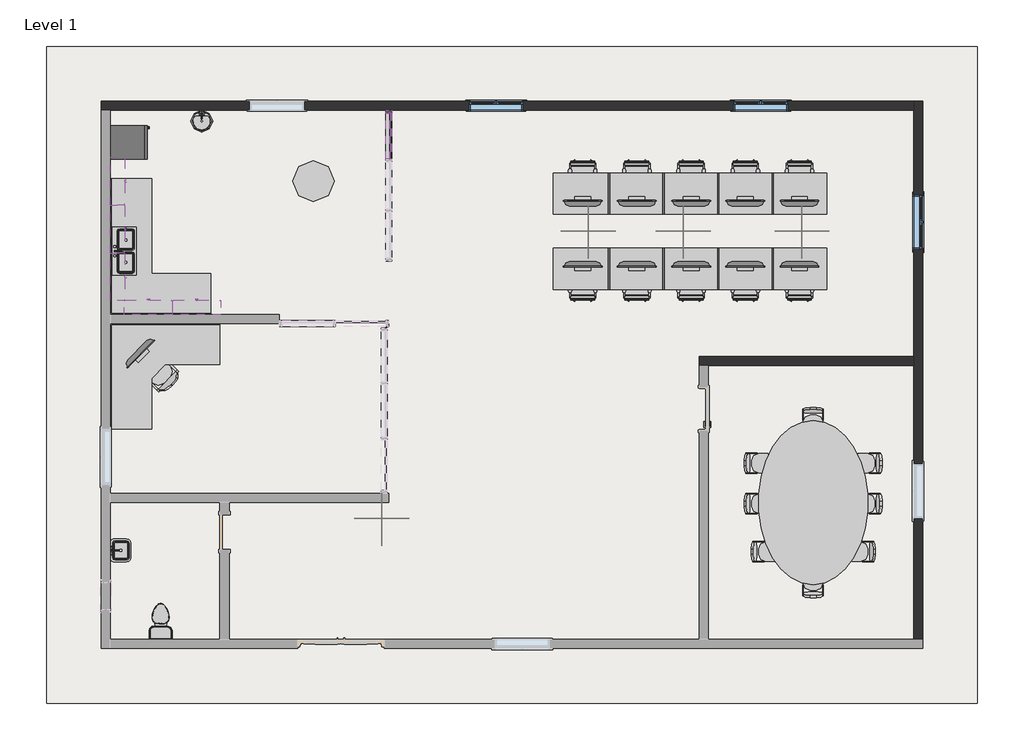
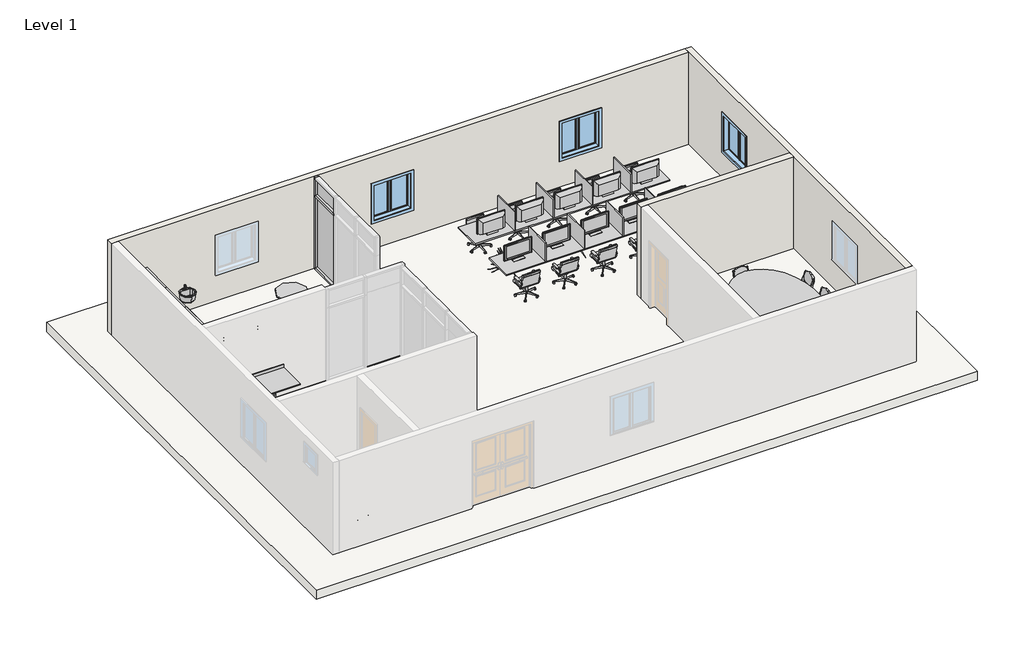
# One storey, part 2 of 2: 43 furniture elements, 10 plates, 4 flow terminals, 4 geographic elements, 4 members, 3 walls, 3 windows, 1 proxy, 1 slab.
"""IFC4 building model written with IfcOpenShell, lengths in millimetres."""

from ifc_helpers import new_model, si_unit, frame, origin, place, context, project, spatial, polyline, outline, extrude, faceted_brep, transform, mapped, element, save
from components import proxy_a13a33b2, flow_terminal_a53be723, flow_terminal_d49f872f, flow_terminal_62a433f7, toilet_domestic_3d_toilet_domestic_3d_f7549cf7, toilet_domestic_3d_toilet_domestic_3d_183bbd19, furniture_2d7fc6e7, chair_executive_chair_executive_8d69e98c, chair_task_arms_chair_task_arms_fa5a08ef, furniture_cfc005fb, furniture_c973ddc6, furniture_51338070, furniture_3d1d9cbc, furniture_2ec127df, furniture_56245f3a, furniture_905aceb5, furniture_1a6705e8, furniture_7e2871f8, rpc_plant_tropical_agave_1_5_74a88192, member_47bfaf8a, member_ee409385, member_a1c24a98, member_38455fd9, system_panel_glazed_82e05715, system_panel_glazed_958d1135, system_panel_glazed_6663e6a9, window_0862ab64

model = new_model("IFC4")

# Units and contexts
model_context = context("Model", 3, world=origin())
ifc_project = project(units=[si_unit("LENGTHUNIT", "METRE", prefix="MILLI")], contexts=[model_context])

# Site, building, storey
site = spatial("IfcSite", under=ifc_project)
building = spatial("IfcBuilding", under=site)
storey = spatial("IfcBuildingStorey", under=building, Name="Level 1", Elevation=0.0)

# Proxy
placement = place(None, origin())
proxy_shape = proxy_a13a33b2(model_context)
element("IfcBuildingElementProxy", 1, Name="Refrigerator : 30\" x 32\" RH", ObjectType="Refrigerator : 30\" x 32\" RH", at=placement, inside=storey, context=model_context, shape_type="MappedRepresentation", body=[
    mapped(proxy_shape, transform((-15846.011402, 5252.7824508, 0.0), x_axis=(0.0, 1.0000000000000002, 0.0), y_axis=(-1.0000000000000002, 0.0, 0.0), z_axis=(0.0, 0.0, 1.0))),
])

# Flow terminals
flow_terminal_shape = flow_terminal_a53be723(model_context)
element("IfcFlowTerminal", 2, ObjectType="Sink Kitchen-Double : 42\" x 21\"", at=placement, inside=storey, context=model_context, shape_type="MappedRepresentation", body=[
    mapped(flow_terminal_shape, transform((-15937.3285008, 2818.9421817, 0.0), x_axis=(0.0, 1.0000000000000002, 0.0), y_axis=(-1.0000000000000002, 0.0, 0.0), z_axis=(0.0, 0.0, 1.0))),
])
flow_terminal_2_shape = flow_terminal_d49f872f(model_context)
element("IfcFlowTerminal", 3, ObjectType="Sink Vanity-Round : 19\" x 19\"", at=placement, inside=storey, context=model_context, shape_type="MappedRepresentation", body=[
    mapped(flow_terminal_2_shape, transform((-14309.1256425, 5647.2327419, 0.0), x_axis=(1.0, 0.0, 0.0), y_axis=(0.0, 1.0, 0.0), z_axis=(0.0, 0.0, 1.0))),
])
flow_terminal_3_shape = flow_terminal_62a433f7(model_context)
element("IfcFlowTerminal", 4, ObjectType="Sink Vanity-Square : 20\" x 18\"", at=placement, inside=storey, context=model_context, shape_type="MappedRepresentation", body=[
    mapped(flow_terminal_3_shape, transform((-16064.3285008, -3848.5578183, 0.0), x_axis=(0.0, 1.0000000000000002, 0.0), y_axis=(-1.0000000000000002, 0.0, 0.0), z_axis=(0.0, 0.0, 1.0))),
])
toilet_domestic_3d_toilet_domestic_3d_shape = toilet_domestic_3d_toilet_domestic_3d_f7549cf7(model_context)
toilet_domestic_3d_toilet_domestic_3d_2_shape = toilet_domestic_3d_toilet_domestic_3d_183bbd19(model_context)
element("IfcFlowTerminal", 5, ObjectType="Toilet-Domestic-3D : Toilet-Domestic-3D", at=placement, inside=storey, context=model_context, shape_type="MappedRepresentation", body=[
    mapped(toilet_domestic_3d_toilet_domestic_3d_shape, transform((-15126.873902, -5319.3725504, 0.0), x_axis=(-1.0000000000000004, 0.0, 0.0), y_axis=(0.0, -1.0000000000000004, 0.0), z_axis=(0.0, 0.0, 1.0))),
    mapped(toilet_domestic_3d_toilet_domestic_3d_2_shape, transform((-15126.873902, -5319.3725504, 0.0), x_axis=(-1.0000000000000004, 0.0, 0.0), y_axis=(0.0, -1.0000000000000004, 0.0), z_axis=(0.0, 0.0, 1.0))),
])

# Furniture
furniture_shape = furniture_2d7fc6e7(model_context)
element("IfcFurniture", 6, ObjectType="48\"", at=placement, inside=storey, context=model_context, shape_type="MappedRepresentation", body=[
    mapped(furniture_shape, transform((-14655.028942, 1424.9314222, 0.0), x_axis=(-1.0000000000000004, 0.0, 0.0), y_axis=(0.0, -1.0000000000000004, 0.0), z_axis=(0.0, 0.0, 1.0))),
])
element("IfcFurniture", 7, ObjectType="48\"", at=placement, inside=storey, context=model_context, shape_type="MappedRepresentation", body=[
    mapped(furniture_shape, transform((-16193.673902, 3772.4864623, 0.0), x_axis=(0.0, 1.0000000000000002, 0.0), y_axis=(-1.0000000000000002, 0.0, 0.0), z_axis=(0.0, 0.0, 1.0))),
])
chair_executive_chair_executive_shape = chair_executive_chair_executive_8d69e98c(model_context)
element("IfcFurniture", 8, ObjectType="Chair-Executive : Chair-Executive", at=placement, inside=storey, context=model_context, shape_type="MappedRepresentation", body=[
    mapped(chair_executive_chair_executive_shape, transform((-15213.1726911, -8.960918, 0.0), x_axis=(0.7071067811865517, 0.707106781186545, 0.0), y_axis=(-0.707106781186545, 0.7071067811865517, 0.0), z_axis=(0.0, 0.0, 1.0))),
])
chair_task_arms_chair_task_arms_shape = chair_task_arms_chair_task_arms_fa5a08ef(model_context)
element("IfcFurniture", 9, ObjectType="Chair-Task Arms : Chair-Task Arms", at=placement, inside=storey, context=model_context, shape_type="MappedRepresentation", body=[
    mapped(chair_task_arms_chair_task_arms_shape, transform((-5587.8830823, 4593.4773239, 0.0), x_axis=(-1.0000000000000004, 0.0, 0.0), y_axis=(0.0, -1.0000000000000004, 0.0), z_axis=(0.0, 0.0, 1.0))),
])
element("IfcFurniture", 10, ObjectType="Chair-Task Arms : Chair-Task Arms", at=placement, inside=storey, context=model_context, shape_type="MappedRepresentation", body=[
    mapped(chair_task_arms_chair_task_arms_shape, transform((-5869.8647216, 1990.1855206, 0.0), x_axis=(1.0000000000000002, 0.0, 0.0), y_axis=(0.0, 1.0000000000000002, 0.0), z_axis=(0.0, 0.0, 1.0))),
])
element("IfcFurniture", 11, ObjectType="Chair-Task Arms : Chair-Task Arms", at=placement, inside=storey, context=model_context, shape_type="MappedRepresentation", body=[
    mapped(chair_task_arms_chair_task_arms_shape, transform((-761.8830823, 4593.4773239, 0.0), x_axis=(-1.0, 0.0, 0.0), y_axis=(0.0, -1.0, 0.0), z_axis=(0.0, 0.0, 1.0))),
])
element("IfcFurniture", 12, ObjectType="Chair-Task Arms : Chair-Task Arms", at=placement, inside=storey, context=model_context, shape_type="MappedRepresentation", body=[
    mapped(chair_task_arms_chair_task_arms_shape, transform((-1043.8647216, 1990.1855206, 0.0), x_axis=(1.0, 0.0, 0.0), y_axis=(0.0, 1.0, 0.0), z_axis=(0.0, 0.0, 1.0))),
])
element("IfcFurniture", 13, ObjectType="Chair-Task Arms : Chair-Task Arms", at=placement, inside=storey, context=model_context, shape_type="MappedRepresentation", body=[
    mapped(chair_task_arms_chair_task_arms_shape, transform((-4381.3830823, 4593.4773239, 0.0), x_axis=(-1.0, 0.0, 0.0), y_axis=(0.0, -1.0, 0.0), z_axis=(0.0, 0.0, 1.0))),
])
element("IfcFurniture", 14, ObjectType="Chair-Task Arms : Chair-Task Arms", at=placement, inside=storey, context=model_context, shape_type="MappedRepresentation", body=[
    mapped(chair_task_arms_chair_task_arms_shape, transform((-4663.3647216, 1990.1855206, 0.0), x_axis=(1.0, 0.0, 0.0), y_axis=(0.0, 1.0, 0.0), z_axis=(0.0, 0.0, 1.0))),
])
element("IfcFurniture", 15, ObjectType="Chair-Task Arms : Chair-Task Arms", at=placement, inside=storey, context=model_context, shape_type="MappedRepresentation", body=[
    mapped(chair_task_arms_chair_task_arms_shape, transform((-3174.8830823, 4593.4773239, 0.0), x_axis=(-1.0, 0.0, 0.0), y_axis=(0.0, -1.0, 0.0), z_axis=(0.0, 0.0, 1.0))),
])
element("IfcFurniture", 16, ObjectType="Chair-Task Arms : Chair-Task Arms", at=placement, inside=storey, context=model_context, shape_type="MappedRepresentation", body=[
    mapped(chair_task_arms_chair_task_arms_shape, transform((-3456.8647216, 1990.1855206, 0.0), x_axis=(1.0, 0.0, 0.0), y_axis=(0.0, 1.0, 0.0), z_axis=(0.0, 0.0, 1.0))),
])
element("IfcFurniture", 17, ObjectType="Chair-Task Arms : Chair-Task Arms", at=placement, inside=storey, context=model_context, shape_type="MappedRepresentation", body=[
    mapped(chair_task_arms_chair_task_arms_shape, transform((-1968.3830823, 4593.4773239, 0.0), x_axis=(-1.0, 0.0, 0.0), y_axis=(0.0, -1.0, 0.0), z_axis=(0.0, 0.0, 1.0))),
])
element("IfcFurniture", 18, ObjectType="Chair-Task Arms : Chair-Task Arms", at=placement, inside=storey, context=model_context, shape_type="MappedRepresentation", body=[
    mapped(chair_task_arms_chair_task_arms_shape, transform((-2250.3647216, 1990.1855206, 0.0), x_axis=(1.0, 0.0, 0.0), y_axis=(0.0, 1.0, 0.0), z_axis=(0.0, 0.0, 1.0))),
])
furniture_2_shape = furniture_cfc005fb(model_context)
element("IfcFurniture", 19, ObjectType="Counter Top-Island : 48\" Depth", at=placement, inside=storey, context=model_context, shape_type="MappedRepresentation", body=[
    mapped(furniture_2_shape, transform((-5188.8116069, 4549.1314222, 914.4), x_axis=(1.0, 0.0, 0.0), y_axis=(0.0, 1.0, 0.0), z_axis=(0.0, 0.0, 1.0))),
])
element("IfcFurniture", 20, ObjectType="Counter Top-Island : 48\" Depth", at=placement, inside=storey, context=model_context, shape_type="MappedRepresentation", body=[
    mapped(furniture_2_shape, transform((-5188.8116069, 2872.7314222, 914.4), x_axis=(1.0, 0.0, 0.0), y_axis=(0.0, 1.0, 0.0), z_axis=(0.0, 0.0, 1.0))),
])
furniture_3_shape = furniture_c973ddc6(model_context)
element("IfcFurniture", 21, ObjectType="Counter Top-L Shaped 2 : 24\" Depth", at=placement, inside=storey, context=model_context, shape_type="MappedRepresentation", body=[
    mapped(furniture_3_shape, transform((-15044.0116069, 1221.7314222, 0.0), x_axis=(1.0, 0.0, 0.0), y_axis=(0.0, 1.0, 0.0), z_axis=(0.0, 0.0, 1.0))),
])
furniture_4_shape = furniture_51338070(model_context)
element("IfcFurniture", 22, ObjectType="Counter Top-L Shaped w Sink : 24\" Depth", at=placement, inside=storey, context=model_context, shape_type="MappedRepresentation", body=[
    mapped(furniture_4_shape, transform((-16244.473902, 2625.3937173, 0.0), x_axis=(0.0, 1.0000000000000002, 0.0), y_axis=(-1.0000000000000002, 0.0, 0.0), z_axis=(0.0, 0.0, 1.0))),
])
furniture_5_shape = furniture_3d1d9cbc(model_context)
element("IfcFurniture", 23, ObjectType="Seating-Auditorium : 18\" x 24\" x 30\"", at=placement, inside=storey, context=model_context, shape_type="MappedRepresentation", body=[
    mapped(furniture_5_shape, transform((-1880.1493118, -3697.5407089, 0.0), x_axis=(0.0, -1.0000000000000004, 0.0), y_axis=(1.0000000000000004, 0.0, 0.0), z_axis=(0.0, 0.0, 1.0))),
])
element("IfcFurniture", 24, ObjectType="Seating-Auditorium : 18\" x 24\" x 30\"", at=placement, inside=storey, context=model_context, shape_type="MappedRepresentation", body=[
    mapped(furniture_5_shape, transform((-2032.5493118, -2630.7407089, 0.0), x_axis=(0.0, -1.0, 0.0), y_axis=(1.0, 0.0, 0.0), z_axis=(0.0, 0.0, 1.0))),
])
element("IfcFurniture", 25, ObjectType="Seating-Auditorium : 18\" x 24\" x 30\"", at=placement, inside=storey, context=model_context, shape_type="MappedRepresentation", body=[
    mapped(furniture_5_shape, transform((-2032.5493118, -1729.0407089, 0.0), x_axis=(0.0, -1.0, 0.0), y_axis=(1.0, 0.0, 0.0), z_axis=(0.0, 0.0, 1.0))),
])
element("IfcFurniture", 26, ObjectType="Seating-Auditorium : 18\" x 24\" x 30\"", at=placement, inside=storey, context=model_context, shape_type="MappedRepresentation", body=[
    mapped(furniture_5_shape, transform((-437.3460331, -747.3931679, 0.0), x_axis=(-1.0000000000000002, 0.0, 0.0), y_axis=(0.0, -1.0000000000000002, 0.0), z_axis=(0.0, 0.0, 1.0))),
])
element("IfcFurniture", 27, ObjectType="Seating-Auditorium : 18\" x 24\" x 30\"", at=placement, inside=storey, context=model_context, shape_type="MappedRepresentation", body=[
    mapped(furniture_5_shape, transform((-758.8017708, -4784.7439876, 0.0), x_axis=(1.0000000000000002, 0.0, 0.0), y_axis=(0.0, 1.0000000000000002, 0.0), z_axis=(0.0, 0.0, 1.0))),
])
furniture_6_shape = furniture_2ec127df(model_context)
element("IfcFurniture", 28, ObjectType="Seating-Auditorium : 18\" x 24\" x 30\"", at=placement, inside=storey, context=model_context, shape_type="MappedRepresentation", body=[
    mapped(furniture_6_shape, transform((684.0015079, -3697.5407089, 0.0), x_axis=(0.0, -1.0000000000000004, 0.0), y_axis=(1.0000000000000004, 0.0, 0.0), z_axis=(0.0, 0.0, 1.0))),
])
element("IfcFurniture", 29, ObjectType="Seating-Auditorium : 18\" x 24\" x 30\"", at=placement, inside=storey, context=model_context, shape_type="MappedRepresentation", body=[
    mapped(furniture_6_shape, transform((836.4015079, -2630.7407089, 0.0), x_axis=(0.0, -1.0, 0.0), y_axis=(1.0, 0.0, 0.0), z_axis=(0.0, 0.0, 1.0))),
])
element("IfcFurniture", 30, ObjectType="Seating-Auditorium : 18\" x 24\" x 30\"", at=placement, inside=storey, context=model_context, shape_type="MappedRepresentation", body=[
    mapped(furniture_6_shape, transform((836.4015079, -1729.0407089, 0.0), x_axis=(0.0, -1.0, 0.0), y_axis=(1.0, 0.0, 0.0), z_axis=(0.0, 0.0, 1.0))),
])
furniture_7_shape = furniture_56245f3a(model_context)
element("IfcFurniture", 31, ObjectType="TV - Flat Screen : 32\"", at=placement, inside=storey, context=model_context, shape_type="MappedRepresentation", body=[
    mapped(furniture_7_shape, transform((-15605.6880737, 588.5239794, 914.4), x_axis=(0.7071067811865503, 0.7071067811865462, 0.0), y_axis=(-0.7071067811865462, 0.7071067811865503, 0.0), z_axis=(0.0, 0.0, 1.0))),
])
element("IfcFurniture", 32, ObjectType="TV - Flat Screen : 32\"", at=placement, inside=storey, context=model_context, shape_type="MappedRepresentation", body=[
    mapped(furniture_7_shape, transform((-5732.8184161, 3898.7406257, 914.4), x_axis=(-1.0000000000000004, 0.0, 0.0), y_axis=(0.0, -1.0000000000000004, 0.0), z_axis=(0.0, 0.0, 1.0))),
])
element("IfcFurniture", 33, ObjectType="TV - Flat Screen : 32\"", at=placement, inside=storey, context=model_context, shape_type="MappedRepresentation", body=[
    mapped(furniture_7_shape, transform((-5724.9293878, 2548.0551491, 914.4), x_axis=(1.0000000000000002, 0.0, 0.0), y_axis=(0.0, 1.0000000000000002, 0.0), z_axis=(0.0, 0.0, 1.0))),
])
element("IfcFurniture", 34, ObjectType="TV - Flat Screen : 32\"", at=placement, inside=storey, context=model_context, shape_type="MappedRepresentation", body=[
    mapped(furniture_7_shape, transform((-906.8184161, 3898.7406257, 914.4), x_axis=(-1.0, 0.0, 0.0), y_axis=(0.0, -1.0, 0.0), z_axis=(0.0, 0.0, 1.0))),
])
element("IfcFurniture", 35, ObjectType="TV - Flat Screen : 32\"", at=placement, inside=storey, context=model_context, shape_type="MappedRepresentation", body=[
    mapped(furniture_7_shape, transform((-898.9293878, 2548.0551491, 914.4), x_axis=(1.0, 0.0, 0.0), y_axis=(0.0, 1.0, 0.0), z_axis=(0.0, 0.0, 1.0))),
])
element("IfcFurniture", 36, ObjectType="TV - Flat Screen : 32\"", at=placement, inside=storey, context=model_context, shape_type="MappedRepresentation", body=[
    mapped(furniture_7_shape, transform((-4526.3184161, 3898.7406257, 914.4), x_axis=(-1.0, 0.0, 0.0), y_axis=(0.0, -1.0, 0.0), z_axis=(0.0, 0.0, 1.0))),
])
element("IfcFurniture", 37, ObjectType="TV - Flat Screen : 32\"", at=placement, inside=storey, context=model_context, shape_type="MappedRepresentation", body=[
    mapped(furniture_7_shape, transform((-4518.4293878, 2548.0551491, 914.4), x_axis=(1.0, 0.0, 0.0), y_axis=(0.0, 1.0, 0.0), z_axis=(0.0, 0.0, 1.0))),
])
element("IfcFurniture", 38, ObjectType="TV - Flat Screen : 32\"", at=placement, inside=storey, context=model_context, shape_type="MappedRepresentation", body=[
    mapped(furniture_7_shape, transform((-3319.8184161, 3898.7406257, 914.4), x_axis=(-1.0, 0.0, 0.0), y_axis=(0.0, -1.0, 0.0), z_axis=(0.0, 0.0, 1.0))),
])
element("IfcFurniture", 39, ObjectType="TV - Flat Screen : 32\"", at=placement, inside=storey, context=model_context, shape_type="MappedRepresentation", body=[
    mapped(furniture_7_shape, transform((-3311.9293878, 2548.0551491, 914.4), x_axis=(1.0, 0.0, 0.0), y_axis=(0.0, 1.0, 0.0), z_axis=(0.0, 0.0, 1.0))),
])
element("IfcFurniture", 40, ObjectType="TV - Flat Screen : 32\"", at=placement, inside=storey, context=model_context, shape_type="MappedRepresentation", body=[
    mapped(furniture_7_shape, transform((-2113.3184161, 3898.7406257, 914.4), x_axis=(-1.0, 0.0, 0.0), y_axis=(0.0, -1.0, 0.0), z_axis=(0.0, 0.0, 1.0))),
])
element("IfcFurniture", 41, ObjectType="TV - Flat Screen : 32\"", at=placement, inside=storey, context=model_context, shape_type="MappedRepresentation", body=[
    mapped(furniture_7_shape, transform((-2105.4293878, 2548.0551491, 914.4), x_axis=(1.0, 0.0, 0.0), y_axis=(0.0, 1.0, 0.0), z_axis=(0.0, 0.0, 1.0))),
])
furniture_8_shape = furniture_905aceb5(model_context)
element("IfcFurniture", 42, ObjectType="Table-Dining Round w Chairs : 36\" Diameter", at=placement, inside=storey, context=model_context, shape_type="MappedRepresentation", body=[
    mapped(furniture_8_shape, transform((-11826.9558692, 4581.6101108, 0.0), x_axis=(1.0, 0.0, 0.0), y_axis=(0.0, 1.0, 0.0), z_axis=(0.0, 0.0, 1.0))),
])
furniture_9_shape = furniture_1a6705e8(model_context)
element("IfcFurniture", 43, ObjectType="Table-Ellipse : 72\" x 36\"", at=placement, inside=storey, context=model_context, shape_type="MappedRepresentation", body=[
    mapped(furniture_9_shape, transform((-598.073902, -2766.0685778, 0.0), x_axis=(0.0, 1.0, 0.0), y_axis=(-1.0, 0.0, 0.0), z_axis=(0.0, 0.0, 1.0))),
])
furniture_10_shape = furniture_7e2871f8(model_context)
element("IfcFurniture", 44, ObjectType="Upper Cabinet-Double Door-Wall : 42\"", at=placement, inside=storey, context=model_context, shape_type="MappedRepresentation", body=[
    mapped(furniture_10_shape, transform((-16346.073902, 2292.902585, 573.9321915), x_axis=(0.0, -1.0, 0.0), y_axis=(1.0, 0.0, 0.0), z_axis=(0.0, 0.0, 1.0))),
])
element("IfcFurniture", 45, ObjectType="Upper Cabinet-Double Door-Wall : 42\"", at=placement, inside=storey, context=model_context, shape_type="MappedRepresentation", body=[
    mapped(furniture_10_shape, transform((-16346.073902, 4426.502585, 573.9321915), x_axis=(0.0, -1.0, 0.0), y_axis=(1.0, 0.0, 0.0), z_axis=(0.0, 0.0, 1.0))),
])
element("IfcFurniture", 46, ObjectType="Upper Cabinet-Double Door-Wall : 42\"", at=placement, inside=storey, context=model_context, shape_type="MappedRepresentation", body=[
    mapped(furniture_10_shape, transform((-16346.073902, 3359.702585, 573.9321915), x_axis=(0.0, -1.0, 0.0), y_axis=(1.0, 0.0, 0.0), z_axis=(0.0, 0.0, 1.0))),
])
element("IfcFurniture", 47, ObjectType="Upper Cabinet-Double Door-Wall : 42\"", at=placement, inside=storey, context=model_context, shape_type="MappedRepresentation", body=[
    mapped(furniture_10_shape, transform((-15429.6950647, 1323.3314222, 588.7403508), x_axis=(1.0, 0.0, 0.0), y_axis=(0.0, 1.0, 0.0), z_axis=(0.0, 0.0, 1.0))),
])
element("IfcFurniture", 48, ObjectType="Upper Cabinet-Double Door-Wall : 42\"", at=placement, inside=storey, context=model_context, shape_type="MappedRepresentation", body=[
    mapped(furniture_10_shape, transform((-14356.5450647, 1323.3314222, 588.7403508), x_axis=(1.0, 0.0, 0.0), y_axis=(0.0, 1.0, 0.0), z_axis=(0.0, 0.0, 1.0))),
])

# Geographic elements
rpc_plant_tropical_agave_1_5_shape = rpc_plant_tropical_agave_1_5_74a88192(model_context)
element("IfcGeographicElement", 49, ObjectType="RPC Plant - Tropical : Agave - 1.5'", at=placement, inside=storey, context=model_context, shape_type="MappedRepresentation", body=[
    mapped(rpc_plant_tropical_agave_1_5_shape, transform((-5606.953902, 3279.1314222, 0.0), x_axis=(1.0, 0.0, 0.0), y_axis=(0.0, 1.0, 0.0), z_axis=(0.0, 0.0, 1.0))),
])
element("IfcGeographicElement", 50, ObjectType="RPC Plant - Tropical : Agave - 1.5'", at=placement, inside=storey, context=model_context, shape_type="MappedRepresentation", body=[
    mapped(rpc_plant_tropical_agave_1_5_shape, transform((-3493.673902, 3279.1314222, 0.0), x_axis=(1.0, 0.0, 0.0), y_axis=(0.0, 1.0, 0.0), z_axis=(0.0, 0.0, 1.0))),
])
element("IfcGeographicElement", 51, ObjectType="RPC Plant - Tropical : Agave - 1.5'", at=placement, inside=storey, context=model_context, shape_type="MappedRepresentation", body=[
    mapped(rpc_plant_tropical_agave_1_5_shape, transform((-852.073902, 3279.1314222, 0.0), x_axis=(1.0, 0.0, 0.0), y_axis=(0.0, 1.0, 0.0), z_axis=(0.0, 0.0, 1.0))),
])
element("IfcGeographicElement", 52, ObjectType="RPC Plant - Tropical : Agave - 1.5'", at=placement, inside=storey, context=model_context, shape_type="MappedRepresentation", body=[
    mapped(rpc_plant_tropical_agave_1_5_shape, transform((-10204.353902, -3121.6685778, 0.0), x_axis=(1.0, 0.0, 0.0), y_axis=(0.0, 1.0, 0.0), z_axis=(0.0, 0.0, 1.0))),
])

# Members
member_shape = member_47bfaf8a(model_context)
element("IfcMember", 53, ObjectType="Rectangular Mullion : 2.5\" x 5\" rectangular", at=placement, inside=storey, context=model_context, shape_type="MappedRepresentation", body=[
    mapped(member_shape, transform((-10046.873902, 5971.5314222, 3048.0), x_axis=(0.0, 1.0, 0.0), y_axis=(-1.0, 0.0, 0.0), z_axis=(0.0, 0.0, 1.0))),
])
member_2_shape = member_ee409385(model_context)
element("IfcMember", 54, ObjectType="Rectangular Mullion : 2.5\" x 5\" rectangular", at=placement, inside=storey, context=model_context, shape_type="MappedRepresentation", body=[
    mapped(member_2_shape, transform((-10046.873902, 5971.5314222, 2438.4), x_axis=(0.0, 1.0, 0.0), y_axis=(-1.0, 0.0, 0.0), z_axis=(0.0, 0.0, 1.0))),
])
member_3_shape = member_a1c24a98(model_context)
element("IfcMember", 55, ObjectType="Rectangular Mullion : 2.5\" x 5\" rectangular", at=placement, inside=storey, context=model_context, shape_type="MappedRepresentation", body=[
    mapped(member_3_shape, transform((-10046.873902, 5908.0314222, 0.0), x_axis=(0.0, 0.0, -1.0), y_axis=(-1.0, 0.0, 0.0), z_axis=(0.0, 1.0, 0.0))),
])
member_4_shape = member_38455fd9(model_context)
element("IfcMember", 56, ObjectType="Rectangular Mullion : 2.5\" x 5\" rectangular", at=placement, inside=storey, context=model_context, shape_type="MappedRepresentation", body=[
    mapped(member_4_shape, transform((-10046.873902, 4885.6814222, 2438.4), x_axis=(0.0, 0.0, 1.0), y_axis=(-1.0, 0.0, 0.0), z_axis=(0.0, -1.0, 0.0))),
])

# Plates
system_panel_glazed_shape = system_panel_glazed_82e05715(model_context)
element("IfcPlate", 57, ObjectType="System Panel : Glazed", at=placement, inside=storey, context=model_context, shape_type="MappedRepresentation", body=[
    mapped(system_panel_glazed_shape, transform((-5175.153902, 4117.3314222, 914.4), x_axis=(0.0, -1.0, 0.0), y_axis=(1.0, 0.0, 0.0), z_axis=(0.0, 0.0, 1.0))),
])
element("IfcPlate", 58, ObjectType="System Panel : Glazed", at=placement, inside=storey, context=model_context, shape_type="MappedRepresentation", body=[
    mapped(system_panel_glazed_shape, transform((-3961.033902, 4117.3314222, 914.4), x_axis=(0.0, -1.0, 0.0), y_axis=(1.0, 0.0, 0.0), z_axis=(0.0, 0.0, 1.0))),
])
element("IfcPlate", 59, ObjectType="System Panel : Glazed", at=placement, inside=storey, context=model_context, shape_type="MappedRepresentation", body=[
    mapped(system_panel_glazed_shape, transform((-2746.913902, 4117.3314222, 914.4), x_axis=(0.0, -1.0, 0.0), y_axis=(1.0, 0.0, 0.0), z_axis=(0.0, 0.0, 1.0))),
])
element("IfcPlate", 60, ObjectType="System Panel : Glazed", at=placement, inside=storey, context=model_context, shape_type="MappedRepresentation", body=[
    mapped(system_panel_glazed_shape, transform((-1532.793902, 4117.3314222, 914.4), x_axis=(0.0, -1.0, 0.0), y_axis=(1.0, 0.0, 0.0), z_axis=(0.0, 0.0, 1.0))),
])
element("IfcPlate", 61, ObjectType="System Panel : Glazed", at=placement, inside=storey, context=model_context, shape_type="MappedRepresentation", body=[
    mapped(system_panel_glazed_shape, transform((-5175.153902, 2440.9314222, 914.4), x_axis=(0.0, -1.0, 0.0), y_axis=(1.0, 0.0, 0.0), z_axis=(0.0, 0.0, 1.0))),
])
element("IfcPlate", 62, ObjectType="System Panel : Glazed", at=placement, inside=storey, context=model_context, shape_type="MappedRepresentation", body=[
    mapped(system_panel_glazed_shape, transform((-3961.033902, 2440.9314222, 914.4), x_axis=(0.0, -1.0, 0.0), y_axis=(1.0, 0.0, 0.0), z_axis=(0.0, 0.0, 1.0))),
])
element("IfcPlate", 63, ObjectType="System Panel : Glazed", at=placement, inside=storey, context=model_context, shape_type="MappedRepresentation", body=[
    mapped(system_panel_glazed_shape, transform((-2746.913902, 2440.9314222, 914.4), x_axis=(0.0, -1.0, 0.0), y_axis=(1.0, 0.0, 0.0), z_axis=(0.0, 0.0, 1.0))),
])
element("IfcPlate", 64, ObjectType="System Panel : Glazed", at=placement, inside=storey, context=model_context, shape_type="MappedRepresentation", body=[
    mapped(system_panel_glazed_shape, transform((-1532.793902, 2440.9314222, 914.4), x_axis=(0.0, -1.0, 0.0), y_axis=(1.0, 0.0, 0.0), z_axis=(0.0, 0.0, 1.0))),
])
system_panel_glazed_2_shape = system_panel_glazed_958d1135(model_context)
element("IfcPlate", 65, ObjectType="System Panel : Glazed", at=placement, inside=storey, context=model_context, shape_type="MappedRepresentation", body=[
    mapped(system_panel_glazed_2_shape, transform((-10046.873902, 5396.8564222, 63.5), x_axis=(0.0, -1.0, 0.0), y_axis=(1.0, 0.0, 0.0), z_axis=(0.0, 0.0, 1.0))),
])
system_panel_glazed_3_shape = system_panel_glazed_6663e6a9(model_context)
element("IfcPlate", 66, ObjectType="System Panel : Glazed", at=placement, inside=storey, context=model_context, shape_type="MappedRepresentation", body=[
    mapped(system_panel_glazed_3_shape, transform((-10046.873902, 5396.8564222, 2470.15), x_axis=(0.0, -1.0, 0.0), y_axis=(1.0, 0.0, 0.0), z_axis=(0.0, 0.0, 1.0))),
])

# Slab
element("IfcSlab", 67, ObjectType="Generic - 12\"", at=placement, inside=storey, context=model_context, shape_type="SweptSolid", body=[
    extrude(outline(polyline([(3059.526098, 7393.9314222), (3059.526098, -7236.4685778), (-17666.873902, -7236.4685778), (-17666.873902, 7393.9314222), (3059.526098, 7393.9314222)])), frame((0.0, 0.0, -304.8), z_axis=(0.0, 0.0, 1.0), x_axis=(1.0, 0.0, 0.0)), (0.0, 0.0, 1.0), 304.8),
])

# Walls
element("IfcWall", 68, ObjectType="Generic - 8\"", at=placement, inside=storey, context=model_context, shape_type="Brep", body=[
    faceted_brep([(-16447.673902, 5971.5314222, 0.0), (-16244.473902, 5971.5314222, 0.0), (1637.126098, 5971.5314222, 0.0), (1637.126098, 5971.5314222, 3048.0), (-16244.473902, 5971.5314222, 3048.0), (-16447.673902, 5971.5314222, 3048.0), (-11926.473902, 5971.5314222, 2133.6), (-11926.473902, 5971.5314222, 914.4), (-13145.673902, 5971.5314222, 914.4), (-13145.673902, 5971.5314222, 2133.6), (-7049.673902, 5971.5314222, 2133.6), (-7049.673902, 5971.5314222, 914.4), (-8268.873902, 5971.5314222, 914.4), (-8268.873902, 5971.5314222, 2133.6), (-1156.873902, 5971.5314222, 2133.6), (-1156.873902, 5971.5314222, 914.4), (-2376.073902, 5971.5314222, 914.4), (-2376.073902, 5971.5314222, 2133.6), (-16447.673902, 6174.7314222, 0.0), (-16447.673902, 6174.7314222, 3048.0), (1637.126098, 6174.7314222, 3048.0), (1637.126098, 6174.7314222, 0.0), (-11926.473902, 6174.7314222, 2133.6), (-13145.673902, 6174.7314222, 2133.6), (-13145.673902, 6174.7314222, 914.4), (-11926.473902, 6174.7314222, 914.4), (-7049.673902, 6174.7314222, 2133.6), (-8268.873902, 6174.7314222, 2133.6), (-8268.873902, 6174.7314222, 914.4), (-7049.673902, 6174.7314222, 914.4), (-1156.873902, 6174.7314222, 2133.6), (-2376.073902, 6174.7314222, 2133.6), (-2376.073902, 6174.7314222, 914.4), (-1156.873902, 6174.7314222, 914.4)], [[[0, 1, 2, 3, 4, 5], [6, 7, 8, 9], [10, 11, 12, 13], [14, 15, 16, 17]], [[18, 19, 20, 21], [22, 23, 24, 25], [26, 27, 28, 29], [30, 31, 32, 33]], [[2, 1, 0, 18, 21]], [[5, 4, 3, 20, 19]], [[0, 5, 19, 18]], [[3, 2, 21, 20]], [[7, 6, 22, 25]], [[8, 7, 25, 24]], [[9, 8, 24, 23]], [[6, 9, 23, 22]], [[11, 10, 26, 29]], [[12, 11, 29, 28]], [[13, 12, 28, 27]], [[10, 13, 27, 26]], [[15, 14, 30, 33]], [[16, 15, 33, 32]], [[17, 16, 32, 31]], [[14, 17, 31, 30]]]),
])
element("IfcWall", 69, ObjectType="Generic - 8\"", at=placement, inside=storey, context=model_context, shape_type="Brep", body=[
    faceted_brep([(1637.126098, 6174.7314222, 0.0), (1637.126098, 5971.5314222, 0.0), (1637.126098, 485.1314222, 0.0), (1637.126098, 281.9314222, 0.0), (1637.126098, -5814.0685778, 0.0), (1637.126098, -5814.0685778, 3048.0), (1637.126098, 281.9314222, 3048.0), (1637.126098, 485.1314222, 3048.0), (1637.126098, 5971.5314222, 3048.0), (1637.126098, 6174.7314222, 3048.0), (1637.126098, 2872.7314222, 2133.6), (1637.126098, 2872.7314222, 914.4), (1637.126098, 4091.9314222, 914.4), (1637.126098, 4091.9314222, 2133.6), (1637.126098, -1902.4685778, 2133.6), (1637.126098, -3121.6685778, 2133.6), (1637.126098, -3121.6685778, 914.4), (1637.126098, -1902.4685778, 914.4), (1840.326098, 6174.7314222, 0.0), (1840.326098, 6174.7314222, 3048.0), (1840.326098, -5814.0685778, 3048.0), (1840.326098, -5814.0685778, 0.0), (1840.326098, 2872.7314222, 2133.6), (1840.326098, 4091.9314222, 2133.6), (1840.326098, 4091.9314222, 914.4), (1840.326098, 2872.7314222, 914.4), (1840.326098, -1902.4685778, 2133.6), (1840.326098, -1902.4685778, 914.4), (1840.326098, -3121.6685778, 914.4), (1840.326098, -3121.6685778, 2133.6)], [[[0, 1, 2, 3, 4, 5, 6, 7, 8, 9], [10, 11, 12, 13], [14, 15, 16, 17]], [[18, 19, 20, 21], [22, 23, 24, 25], [26, 27, 28, 29]], [[4, 3, 2, 1, 0, 18, 21]], [[9, 8, 7, 6, 5, 20, 19]], [[0, 9, 19, 18]], [[5, 4, 21, 20]], [[11, 10, 22, 25]], [[12, 11, 25, 24]], [[13, 12, 24, 23]], [[10, 13, 23, 22]], [[27, 26, 14, 17]], [[28, 27, 17, 16]], [[29, 28, 16, 15]], [[26, 29, 15, 14]]]),
])
element("IfcWall", 70, ObjectType="Generic - 8\"", at=placement, inside=storey, context=model_context, shape_type="Brep", body=[
    faceted_brep([(1637.126098, 485.1314222, 0.0), (-3138.073902, 485.1314222, 0.0), (-3138.073902, 485.1314222, 3048.0), (1637.126098, 485.1314222, 3048.0), (1637.126098, 281.9314222, 0.0), (1637.126098, 281.9314222, 3048.0), (-2934.873902, 281.9314222, 3048.0), (-3138.073902, 281.9314222, 3048.0), (-3138.073902, 281.9314222, 0.0), (-2934.873902, 281.9314222, 0.0)], [[[0, 1, 2, 3]], [[4, 5, 6, 7, 8, 9]], [[1, 0, 4, 9, 8]], [[3, 2, 7, 6, 5]], [[0, 3, 5, 4]], [[2, 1, 8, 7]]]),
])

# Windows
window_shape = window_0862ab64(model_context)
element("IfcWindow", 71, ObjectType="Casement Dbl with Trim : 48\" x 48\"", at=placement, inside=storey, context=model_context, shape_type="MappedRepresentation", body=[
    mapped(window_shape, transform((-7659.273902, 6054.0814222, 0.0), x_axis=(1.0, 0.0, 0.0), y_axis=(0.0, 1.0, 0.0), z_axis=(0.0, 0.0, 1.0))),
])
element("IfcWindow", 72, ObjectType="Casement Dbl with Trim : 48\" x 48\"", at=placement, inside=storey, context=model_context, shape_type="MappedRepresentation", body=[
    mapped(window_shape, transform((-1766.473902, 6054.0814222, 0.0), x_axis=(1.0, 0.0, 0.0), y_axis=(0.0, 1.0, 0.0), z_axis=(0.0, 0.0, 1.0))),
])
element("IfcWindow", 73, ObjectType="Casement Dbl with Trim : 48\" x 48\"", at=placement, inside=storey, context=model_context, shape_type="MappedRepresentation", body=[
    mapped(window_shape, transform((1719.676098, 3482.3314222, 0.0), x_axis=(0.0, -1.0, 0.0), y_axis=(1.0, 0.0, 0.0), z_axis=(0.0, 0.0, 1.0))),
])

save(model, "model.ifc")

# Revit data of these elements
# Type "Refrigerator : 30\" x 32\" RH"
#   Label = "REF."
#   Assembly Code = "E1090400"
#   Depth = 2' - 7 3/4"
#   Handle = 2' - 3"
#   Height = 5' - 10"
#   Rear Clearance = 0' - 2"
#   Top Door Height = 1' - 8"
#   Width = 2' - 5 3/8"
#   Material = Steel, Paint Finish, Ivory, Glossy
#   Default Elevation = 0
# Type "Sink Kitchen-Double : 42\" x 21\""
#   Assembly Code = "D2010410"
#   Counter Height = 3' - 0"
#   Depth = 1' - 9"
#   Width = 3' - 6"
#   Faucet Material = Steel, Polished
#   Sink Material = Steel, Polished
#   Default Elevation = 0
# Type "Sink Vanity-Round : 19\" x 19\""
#   Assembly Code = "D2010400"
#   Top Of Counter = 2' - 7"
#   Basin Material = Porcelain, Linen
#   Faucet Material = Steel, Polished
#   Default Elevation = 0
# Type "Sink Vanity-Square : 20\" x 18\""
#   Assembly Code = "D2010400"
#   Counter Height = 2' - 7"
#   Depth = 1' - 6"
#   Width = 1' - 8"
#   Basin Material = Porcelain, Linen
#   Faucet Material = Steel, Polished
#   Default Elevation = 0
# Type "Toilet-Domestic-3D : Toilet-Domestic-3D"
#   Assembly Code = "D2010110"
#   Toilet - Bowl/Basin Material = Porcelain, Linen
#   Toilet - Seat Material = Laminate, Linen, Matte
#   Default Elevation = 0
# Type "48\""
#   Assembly Code = "C1030410"
#   Depth = 2' - 9"
#   Height = 2' - 9"
#   Toe Depth = 0' - 3"
#   Toe Height = 0' - 3 1/2"
#   Width = 3' - 8"
#   Cabinet Material = none
#   Door/Drawer Material = none
#   Handle Material = Cabinets - Handles
#   Default Elevation = 0
# Type "Chair-Executive : Chair-Executive"
#   Assembly Code = "E2020200"
#   Base/Arms Material = Plastic, Opaque Black
#   Casters Material = Plastic, Opaque Black
#   Seat/Back Material = Textile - Slate Blue
#   Default Elevation = 0
# Type "Chair-Task Arms : Chair-Task Arms"
#   Assembly Code = "E2020200"
#   Base Material = Plastic, Opaque Black
#   Caster Material = Plastic, Opaque Black
#   Seat/Back Material = Textile - Slate Blue
#   Default Elevation = 0
# Type "Counter Top-Island : 48\" Depth"
#   Assembly Code = "C1030400"
#   Width = 3' - 0"
#   Counter Thickness = 0' - 1 1/2"
#   Depth [instance default] = 4' - 2"
#   Length [instance default] = 8' - 0"
#   Counter Top Material = none
#   Default Elevation = 0
#   Height = 0
# Type "Counter Top-L Shaped 2 : 24\" Depth"
#   Assembly Code = "C1030400"
#   Counter Thickness = 0' - 1 1/2"
#   Depth = 3' - 0"
#   Height = 3' - 0"
#   Length - Leg 1 [instance default] = 8' - 0"
#   Length - Leg 2 [instance default] = 6' - 0"
#   Counter Top Material = none
#   Default Elevation = 0
# Type "Counter Top-L Shaped w Sink : 24\" Depth"
#   Assembly Code = "C1030400"
#   Counter Thickness = 0' - 1 1/2"
#   Depth = 3' - 0"
#   Height = 3' - 0"
#   Length - Leg 1 [instance default] = 8' - 0"
#   Length - Leg 2 [instance default] = 6' - 0"
#   Sink Location [instance default] = 3' - 0"
#   Sink Location To Wall [instance default] = 0' - 6"
#   Sink Opening Depth [instance default] = 1' - 3"
#   Sink Opening Width [instance default] = 3' - 3"
#   Counter Top Material = none
#   Default Elevation = 0
# Type "Seating-Auditorium : 18\" x 24\" x 30\""
#   Assembly Code = "E2020200"
#   Seat Material = Linen, Beige
#   Frame Material = Steel, Paint Finish, Dark Gray, Matte
#   Default Elevation = 0
# Type "TV - Flat Screen : 32\""
#   SinAng = 0' - 0.0193"
#   L = 2' - 3.79372"
#   H = 1' - 3.6354"
#   Thickness = 0' - 4.33071"
#   Diagonal = 2' - 7.88976"
#   CosAng = 0' - 0.03431"
#   Stand [instance default] = yes
#   Default Elevation = 0
# Type "Table-Dining Round w Chairs : 36\" Diameter"
#   Assembly Code = "E2020200"
#   Radius = 1' - 6"
#   Diameter = 3' - 0"
#   Height = 2' - 6"
#   Chairs = 4
#   Base Material = Pine
#   Top Material = Laminate, Linen, Matte
#   Default Elevation = 0
# Type "Table-Ellipse : 72\" x 36\""
#   Assembly Code = "E2020200"
#   Half Width = 4' - 0"
#   Half Length = 6' - 0"
#   Height = 2' - 6"
#   Length = 12' - 0"
#   Width = 8' - 0"
#   Base Material = Birch
#   Top Material = Laminate - Black
#   Default Elevation = 0
# Type "Upper Cabinet-Double Door-Wall : 42\""
#   Assembly Code = "C1030410"
#   Depth = 1' - 0"
#   Height = 2' - 6"
#   Top Of Cabinet = 7' - 0"
#   Width = 3' - 6"
#   Cabinet Material = none
#   Door/Drawer Material = none
#   Handle Material = Cabinets - Handles
#   Default Elevation = 0
# Type "RPC Plant - Tropical : Agave - 1.5'"
#   built-in parameter 1005198 = "{2, 15},{39, RPC-16-G1GJ-63FX-7K5P-N000-ST1L-LVER-AU},{1, 0},{1, 0},{2, 13},{1, 8},{5, Color},{1, 0},{1, 0},{3, 0.8},{3, 0.8},{3, 0.8},{1, 8},{7, BBoxMin},{1, 0},{1, 0},{1, 0},{1, 0},{1, 0},{1, 8},{7, BBoxMax},{1, 0},{1, 0},{1, 0},{1, 0},{1, 0},{2, 11},{9, RPCTypeId},{1, 0},{1, 0},{39, RPC-16-G1GJ-63FX-7K5P-N000-ST1L-LVER-AU},{1, 6},{14, RPCPlantHeight},{1, 0},{1, 0},{3, 1.5},{2, 11},{7, keyword},{1, 0},{1, 0},{35, :RPCs:Plants [General]:Geometry:RPC},{2, 11},{8, category},{1, 0},{1, 0},{16, Plants [General]},{2, 11},{12, LocalizedUID},{1, 0},{1, 0},{5, Agave},{2, 14},{6, Height},{1, 0},{1, 0},{3, 1.5},{1, 2},{16, Cast Reflections},{1, 0},{1, 0},{1, 0},{1, 2},{12, Cast Shadows},{1, 0},{1, 0},{1, 1},{1, 2},{9, Lock View},{1, 0},{1, 0},{1, 0},{1, 4},{5, ViewC},{1, 0},{1, 0},{1, 0},{21, assetlibrary_base.fbx},{1, 5},"
#   built-in parameter 1005195 = "RPC-16-G1GJ-63FX-7K5P-N000-ST1L-LVER-AU"
#   Type Comments = "Agave"
#   Assembly Code = "G2050500"
#   Height = 2' - 0"
#   Default Elevation = 0
# Type "Rectangular Mullion : 2.5\" x 5\" rectangular"
#   built-in parameter 1007304 = 0.416667 (stored number, unit not read)
#   built-in parameter 1007301 = 0.104167 (stored number, unit not read)
#   built-in parameter 1007300 = 0.104167 (stored number, unit not read)
# Type "System Panel : Glazed"
#   Construction Type Id = "GSP4R"
#   Analytic Construction = "1/8 in Pilkington single glazing"
#   Visual Light Transmittance = 0.9
#   Solar Heat Gain Coefficient = 0.86
#   Heat Transfer Coefficient (U) = 1.18115 BTU/(h·ft²·°F)
# Type "Generic - 12\""
#   Assembly Code = "B1010"
#   Function = 0
#   Layers, outside or top first: 1' - 0" "FLOOR 1" (function 1)
# Type "Generic - 8\""
#   Assembly Code = "B2010"
#   Layers, outside or top first: 0' - 8" "WALL 1" (function 1)
# Type "Casement Dbl with Trim : 48\" x 48\""
#   Type Mark = "10"
#   Construction Type Id = "GSP4R"
#   Assembly Code = "B2020100"
#   Analytic Construction = "1/8 in Pilkington single glazing"
#   Visual Light Transmittance = 0.9
#   Solar Heat Gain Coefficient = 0.78
#   Heat Transfer Coefficient (U) = 0.6496 BTU/(h·ft²·°F)
#   Height = 4' - 0"
#   Default Sill Height = 3' - 0"
#   Trim Projection - Ext. = 0' - 0 1/2"
#   Trim Projection - Int. = 0' - 0 3/4"
#   Trim Width - Exterior = 0' - 3 1/2"
#   Trim Width - Interior = 0' - 3 1/2"
#   Width = 4' - 0"
#   Window Inset = 0' - 0 3/4"
#   Define Thermal Properties by = 1
#   Glass Pane Material = Glass
#   Sash Material = Sash
#   Trim Exterior Material = Trim
#   Trim Interior Material = Trim
#   Wall Closure = (empty or 0)
# Element 1 (IfcBuildingElementProxy, "Refrigerator : 30\" x 32\" RH")
#   Phase Created = New Construction
#   Materials on its faces: "Steel, Paint Finish, Ivory, Glossy", "Steel, Chrome Plated"
# Element 2 (IfcFlowTerminal, "Sink Kitchen-Double : 42\" x 21\"")
#   Mark = "3"
#   Phase Created = New Construction
#   Materials on its faces: "Steel, Polished"
# Element 3 (IfcFlowTerminal, "Sink Vanity-Round : 19\" x 19\"")
#   Mark = "4"
#   Phase Created = New Construction
#   Materials on its faces: "Porcelain, Linen", "Steel, Polished"
# Element 4 (IfcFlowTerminal, "Sink Vanity-Square : 20\" x 18\"")
#   Mark = "2"
#   Phase Created = New Construction
#   Materials on its faces: "Porcelain, Linen", "Steel, Polished"
# Element 5 (IfcFlowTerminal, "Toilet-Domestic-3D : Toilet-Domestic-3D")
#   Mark = "1"
#   Phase Created = New Construction
#   Materials on its faces: "Porcelain, Linen", "Laminate, Linen, Matte"
# Elements 6, 7 (IfcFurniture, "48\"")
#   Phase Created = New Construction
#   Materials on its faces: "Cabinets", "Cabinets - Handles"
# Element 8 (IfcFurniture, "Chair-Executive : Chair-Executive")
#   Phase Created = New Construction
#   Materials on its faces: "Plastic, Opaque Black", "Textile - Slate Blue"
# Elements 9, 10, 11, 12, 13, 14, 15, 16, 17, 18 (IfcFurniture, "Chair-Task Arms : Chair-Task Arms")
#   Phase Created = New Construction
#   Materials on its faces: "Plastic, Opaque Black", "Textile - Slate Blue"
# Elements 19, 20 (IfcFurniture, "Counter Top-Island : 48\" Depth")
#   Length = 20' - 0"
#   Depth = 3' - 0"
#   Phase Created = New Construction
#   Materials on its faces: "Counter Top"
# Element 21 (IfcFurniture, "Counter Top-L Shaped 2 : 24\" Depth")
#   Length - Leg 2 = 7' - 8.41463"
#   Length - Leg 1 = 8' - 0"
#   Phase Created = New Construction
#   Materials on its faces: "Counter Top"
# Element 22 (IfcFurniture, "Counter Top-L Shaped w Sink : 24\" Depth")
#   Sink Opening Width = 3' - 3"
#   Sink Opening Depth = 1' - 3"
#   Sink Location To Wall = 0' - 6"
#   Sink Location = 3' - 0"
#   Length - Leg 2 = 7' - 4.05203"
#   Length - Leg 1 = 9' - 11.04567"
#   Phase Created = New Construction
#   Materials on its faces: "Counter Top"
# Elements 23, 24, 25, 26, 27, 28, 29, 30 (IfcFurniture, "Seating-Auditorium : 18\" x 24\" x 30\"")
#   Phase Created = New Construction
#   Materials on its faces: "Steel, Paint Finish, Dark Gray, Matte", "Linen, Beige"
# Elements 31, 32, 33, 34, 35, 36, 37, 38, 39, 40, 41 (IfcFurniture, "TV - Flat Screen : 32\"")
#   Stand = yes
#   Phase Created = New Construction
#   Materials on its faces: "TV - Black", "TV - Glass", "TV - Screen"
# Element 42 (IfcFurniture, "Table-Dining Round w Chairs : 36\" Diameter")
#   Phase Created = New Construction
#   Materials on its faces: "Pine", "Laminate, Linen, Matte"
# Element 43 (IfcFurniture, "Table-Ellipse : 72\" x 36\"")
#   Phase Created = New Construction
#   Materials on its faces: "Birch", "Laminate - Black"
# Elements 44, 45, 46, 47, 48 (IfcFurniture, "Upper Cabinet-Double Door-Wall : 42\"")
#   Phase Created = New Construction
#   Materials on its faces: "Cabinets - Handles", "Cabinets"
# Elements 49, 50, 51, 52 (IfcGeographicElement, "RPC Plant - Tropical : Agave - 1.5'")
#   Phase Created = New Construction
# Elements 53, 54, 55, 56 (IfcMember, "Rectangular Mullion : 2.5\" x 5\" rectangular")
#   Phase Created = New Construction
#   Materials on its faces: "Aluminum"
# Elements 57, 58, 59, 60, 61, 62, 63, 64, 65, 66 (IfcPlate, "System Panel : Glazed")
#   Phase Created = New Construction
#   Materials on its faces: "Glass"
# Element 67 (IfcSlab, "Generic - 12\"")
#   Height Offset From Level = 0' - 0"
#   Phase Created = New Construction
#   Materials on its faces: "FLOOR 1"
# Elements 68, 69, 70 (IfcWall, "Generic - 8\"")
#   Top Offset = 0' - 0"
#   Base Offset = 0' - 0"
#   Unconnected Height = 10' - 0"
#   wall height = 10' - 0"
#   Phase Created = New Construction
#   Base Constraint = Level 1
#   Materials on its faces: "WALL 1"
# Element 71 (IfcWindow, "Casement Dbl with Trim : 48\" x 48\"")
#   Mark = "2"
#   Phase Created = New Construction
#   Materials on its faces: "Sash", "Trim", "Glass"
# Element 72 (IfcWindow, "Casement Dbl with Trim : 48\" x 48\"")
#   Mark = "3"
#   Phase Created = New Construction
#   Materials on its faces: "Sash", "Trim", "Glass"
# Element 73 (IfcWindow, "Casement Dbl with Trim : 48\" x 48\"")
#   Mark = "4"
#   Phase Created = New Construction
#   Materials on its faces: "Sash", "Trim", "Glass"
# Materials
#   "Steel, Paint Finish, Ivory, Glossy": class "Metal", colour RGB 247 247 239, transparency 0, Description = "Steel, paint finish, ivory, glossy", Cost = 0
#   "Steel, Polished": class "Metal", colour RGB 57 57 57, transparency 0, Description = "Polished steel", Cost = 0
#   "Porcelain, Linen": class "Ceramic", colour RGB 249 239 230, transparency 0, Description = "Porcelain, linen", Cost = 0
#   "Laminate, Linen, Matte": class "Plastic", colour RGB 249 239 230, transparency 0, Description = "Plastic Laminate - Linen, Matte", Cost = 0
#   "Cabinets - Handles": class "Metal", colour RGB 57 57 57, transparency 0
#   "Plastic, Opaque Black": class "Plastic", colour RGB 0 0 0, transparency 0, Description = "Plastic, generic, opaque black", Cost = 0
#   "Textile - Slate Blue": class "Fabric", colour RGB 98 102 118, transparency 0
#   "Linen, Beige": class "Textile", colour RGB 249 239 230, transparency 0, Description = "Linen, beige", Cost = 0
#   "Steel, Paint Finish, Dark Gray, Matte": class "Metal", colour RGB 0 0 0, transparency 0, Description = "Steel, paint finish, dark gray, matte", Cost = 0
#   "Pine": class "Wood", colour RGB 223 192 134, transparency 0, Description = "Pinus Echinata", Cost = 0
#   "Birch": class "Wood", colour RGB 224 178 126, transparency 0, Description = "Betula Alleghaniensis", Cost = 0
#   "Laminate - Black": colour RGB 0 0 0, transparency 0
#   "FLOOR 1": class "Generic", colour RGB 120 120 120, transparency 0, Cost = 0
#   "WALL 1": class "Generic", colour RGB 120 120 120, transparency 0, Cost = 0
#   "Glass": class "Glass", colour RGB 0 128 192, transparency 0.75, Description = "Soda Lime Glass", Cost = 0
#   "Sash": class "Wood", colour RGB 224 178 126, transparency 0
#   "Trim": class "Wood", colour RGB 224 178 126, transparency 0
#   "Steel, Chrome Plated": class "Metal", colour RGB 17 17 17, transparency 0, Description = "Chromiuim plated steel", Cost = 0
#   "Cabinets": colour RGB 249 249 249, transparency 0
#   "Counter Top": class "Wood", colour RGB 226 177 128, transparency 0
#   "TV - Black": colour RGB 49 49 49, transparency 0
#   "TV - Glass": colour RGB 157 157 157, transparency 0.9
#   "TV - Screen": colour RGB 0 0 0, transparency 0
#   "Aluminum": class "Metal", colour RGB 247 247 247, transparency 0, Description = "Aluminum 6061", Cost = 0
